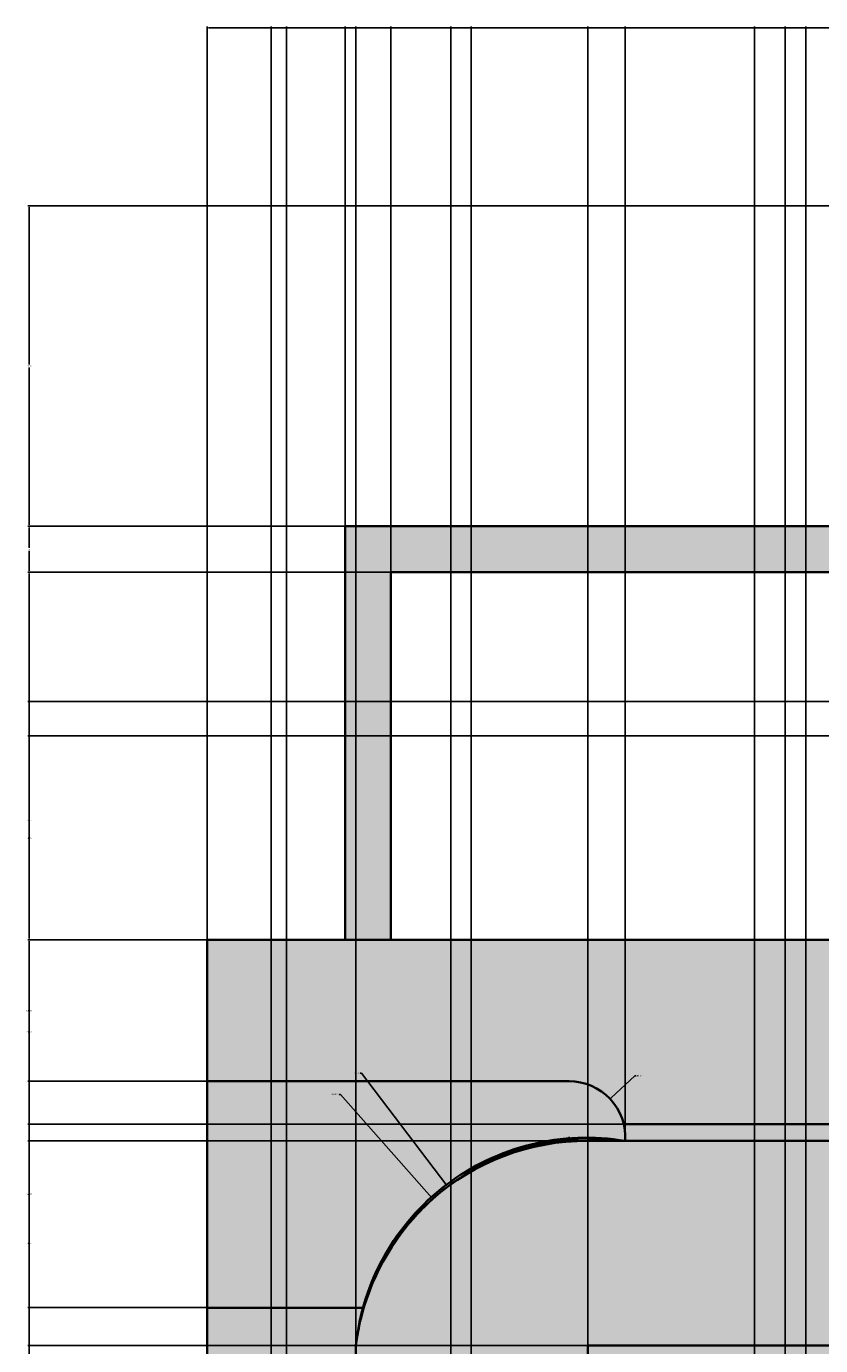
# Model space of a CAD drawing. Units: feet. Extents: x 2368 to 2738, y 1285 to 1782.
# Tile 3 of 6: x 2368 to 2472, y 1610 to 1782. Entities that reach past the tile are written whole.
import ezdxf

# ---------------------------------------------------------------- set-up
doc = ezdxf.new("R2010")
doc.units = ezdxf.units.FT
for name, color, linetype, lineweight in [('A-ANNO-DIMS', 2, 'Continuous', 18), ('A-ELEV', 7, 'Continuous', 35), ('A-ELEV-PATT', 252, 'Continuous', 13)]:
    doc.layers.add(name, color=color, linetype=linetype, lineweight=lineweight)
doc.styles.get("Standard").update_dxf_attribs({"font": 'arial.ttf'})
doc.dimstyles.get("Standard").update_dxf_attribs({"dimtxt": 0.18, "dimasz": 0.18, "dimexe": 0.18, "dimexo": 0.0625, "dimgap": 0.09, "dimtad": 0, "dimtih": 1, "dimtoh": 1, "dimdec": 1, "dimzin": 0, "dimdsep": 46, "dimlunit": 3, "dimtxsty": 'Standard', "dimcen": 0.09, "dimadec": 0, "dimazin": 0, "dimtfac": 1, "dimtdec": 1, "dimtofl": 0, "dimtmove": 0, "dimatfit": 3, "dimfxl": 1, "dimtolj": 1, "dimtzin": 0, "dimarcsym": 0})

# ---------------------------------------------------------------- blocks, each defined once
blk = doc.blocks.new('*D1')
at = {"layer": 'A-ANNO-DIMS', "color": 0, "lineweight": -2, "transparency": 16777216}
for p, q in [((2391.54, 1662.92), (2391.54, 1782.11)), ((2391.72, 1781.93), (2552.46, 1781.93)), ((2713.98, 1781.93), (2553.25, 1781.93)), ((2714.16, 1758.74), (2714.16, 1782.11))]:
    blk.add_line(p, q, dxfattribs=at)
at = {"layer": 'A-ANNO-DIMS', "color": 0, "transparency": 16777216}
for points in [[(2391.72, 1781.96), (2391.72, 1781.9), (2391.54, 1781.93)], [(2713.98, 1781.96), (2713.98, 1781.9), (2714.16, 1781.93)]]:
    blk.add_solid(points, dxfattribs=at)
at = {"layer": 'Defpoints', "color": 0, "transparency": 16777216}
for p in [(2714.16, 1781.93), (2714.16, 1758.68), (2391.54, 1662.86)]:
    blk.add_point(p, dxfattribs=at)
at = {"layer": 'A-ANNO-DIMS', "color": 0, "transparency": 16777216, "insert": (2552.85, 1781.93), "char_height": 0.18, "attachment_point": 5}
blk.add_mtext('\\A1;322.6', dxfattribs=at)
blk = doc.blocks.new('*D8')
at = {"layer": 'A-ANNO-DIMS', "color": 0, "lineweight": -2, "transparency": 16777216}
for p, q in [((2391.48, 1614.86), (2368.11, 1614.86)), ((2368.29, 1614.68), (2368.29, 1552.04)), ((2368.29, 1489.04), (2368.29, 1551.67)), ((2391.48, 1488.86), (2368.11, 1488.86))]:
    blk.add_line(p, q, dxfattribs=at)
at = {"layer": 'A-ANNO-DIMS', "color": 0, "transparency": 16777216}
for points in [[(2368.26, 1614.68), (2368.32, 1614.68), (2368.29, 1614.86)], [(2368.26, 1489.04), (2368.32, 1489.04), (2368.29, 1488.86)]]:
    blk.add_solid(points, dxfattribs=at)
at = {"layer": 'Defpoints', "color": 0, "transparency": 16777216}
for p in [(2368.29, 1614.86), (2391.54, 1614.86), (2391.54, 1488.86)]:
    blk.add_point(p, dxfattribs=at)
at = {"layer": 'A-ANNO-DIMS', "color": 0, "transparency": 16777216, "insert": (2368.29, 1551.86), "char_height": 0.18, "attachment_point": 5}
blk.add_mtext('\\A1;126', dxfattribs=at)
blk = doc.blocks.new('*D9')
at = {"layer": 'A-ANNO-DIMS', "color": 0, "lineweight": -2, "transparency": 16777216}
for p, q in [((2391.48, 1644.42), (2368.11, 1644.42)), ((2368.29, 1644.24), (2368.29, 1629.82)), ((2368.29, 1615.04), (2368.29, 1629.46)), ((2391.48, 1614.86), (2368.11, 1614.86))]:
    blk.add_line(p, q, dxfattribs=at)
at = {"layer": 'A-ANNO-DIMS', "color": 0, "transparency": 16777216}
for points in [[(2368.26, 1644.24), (2368.32, 1644.24), (2368.29, 1644.42)], [(2368.26, 1615.04), (2368.32, 1615.04), (2368.29, 1614.86)]]:
    blk.add_solid(points, dxfattribs=at)
at = {"layer": 'Defpoints', "color": 0, "transparency": 16777216}
for p in [(2368.29, 1644.42), (2391.54, 1644.42), (2391.54, 1614.86)]:
    blk.add_point(p, dxfattribs=at)
at = {"layer": 'A-ANNO-DIMS', "color": 0, "transparency": 16777216, "insert": (2368.29, 1629.64), "char_height": 0.18, "attachment_point": 5}
blk.add_mtext('\\A1;29.565', dxfattribs=at)
blk = doc.blocks.new('*D10')
at = {"layer": 'A-ANNO-DIMS', "color": 0, "lineweight": -2, "transparency": 16777216}
for p, q in [((2391.48, 1662.86), (2368.11, 1662.86)), ((2368.29, 1662.68), (2368.29, 1653.82)), ((2368.29, 1644.6), (2368.29, 1653.46)), ((2391.48, 1644.42), (2368.11, 1644.42))]:
    blk.add_line(p, q, dxfattribs=at)
at = {"layer": 'A-ANNO-DIMS', "color": 0, "transparency": 16777216}
for points in [[(2368.26, 1662.68), (2368.32, 1662.68), (2368.29, 1662.86)], [(2368.26, 1644.6), (2368.32, 1644.6), (2368.29, 1644.42)]]:
    blk.add_solid(points, dxfattribs=at)
at = {"layer": 'Defpoints', "color": 0, "transparency": 16777216}
for p in [(2368.29, 1662.86), (2391.54, 1662.86), (2391.54, 1644.42)]:
    blk.add_point(p, dxfattribs=at)
at = {"layer": 'A-ANNO-DIMS', "color": 0, "transparency": 16777216, "insert": (2368.29, 1653.64), "char_height": 0.18, "attachment_point": 5}
blk.add_mtext('\\A1;18.435', dxfattribs=at)
blk = doc.blocks.new('*D11')
at = {"layer": 'A-ANNO-DIMS', "color": 0, "lineweight": -2, "transparency": 16777216}
for p, q in [((2415.48, 1710.86), (2368.11, 1710.86)), ((2368.29, 1710.68), (2368.29, 1687.04)), ((2368.29, 1663.04), (2368.29, 1686.67)), ((2409.48, 1662.86), (2368.11, 1662.86))]:
    blk.add_line(p, q, dxfattribs=at)
at = {"layer": 'A-ANNO-DIMS', "color": 0, "transparency": 16777216}
for points in [[(2368.26, 1710.68), (2368.32, 1710.68), (2368.29, 1710.86)], [(2368.26, 1663.04), (2368.32, 1663.04), (2368.29, 1662.86)]]:
    blk.add_solid(points, dxfattribs=at)
at = {"layer": 'Defpoints', "color": 0, "transparency": 16777216}
for p in [(2368.29, 1710.86), (2415.54, 1710.86), (2409.54, 1662.86)]:
    blk.add_point(p, dxfattribs=at)
at = {"layer": 'A-ANNO-DIMS', "color": 0, "transparency": 16777216, "insert": (2368.29, 1686.86), "char_height": 0.18, "attachment_point": 5}
blk.add_mtext('\\A1;48', dxfattribs=at)
blk = doc.blocks.new('*D12')
at = {"layer": 'A-ANNO-DIMS', "color": 0, "lineweight": -2, "transparency": 16777216}
for p, q in [((2409.48, 1716.86), (2368.11, 1716.86)), ((2368.29, 1716.68), (2368.29, 1714.04)), ((2368.29, 1711.04), (2368.29, 1713.67)), ((2415.48, 1710.86), (2368.11, 1710.86))]:
    blk.add_line(p, q, dxfattribs=at)
at = {"layer": 'A-ANNO-DIMS', "color": 0, "transparency": 16777216}
for points in [[(2368.26, 1716.68), (2368.32, 1716.68), (2368.29, 1716.86)], [(2368.26, 1711.04), (2368.32, 1711.04), (2368.29, 1710.86)]]:
    blk.add_solid(points, dxfattribs=at)
at = {"layer": 'Defpoints', "color": 0, "transparency": 16777216}
for p in [(2368.29, 1716.86), (2409.54, 1716.86), (2415.54, 1710.86)]:
    blk.add_point(p, dxfattribs=at)
at = {"layer": 'A-ANNO-DIMS', "color": 0, "transparency": 16777216, "insert": (2368.29, 1713.86), "char_height": 0.18, "attachment_point": 5}
blk.add_mtext('\\A1;6', dxfattribs=at)
blk = doc.blocks.new('*D13')
at = {"layer": 'A-ANNO-DIMS', "color": 0, "lineweight": -2, "transparency": 16777216}
for p, q in [((2519.56, 1758.68), (2368.11, 1758.68)), ((2368.29, 1758.5), (2368.29, 1737.95)), ((2368.29, 1717.04), (2368.29, 1737.58)), ((2519.56, 1716.86), (2368.11, 1716.86))]:
    blk.add_line(p, q, dxfattribs=at)
at = {"layer": 'A-ANNO-DIMS', "color": 0, "transparency": 16777216}
for points in [[(2368.26, 1758.5), (2368.32, 1758.5), (2368.29, 1758.68)], [(2368.26, 1717.04), (2368.32, 1717.04), (2368.29, 1716.86)]]:
    blk.add_solid(points, dxfattribs=at)
at = {"layer": 'Defpoints', "color": 0, "transparency": 16777216}
for p in [(2368.29, 1758.68), (2519.62, 1758.68), (2519.62, 1716.86)]:
    blk.add_point(p, dxfattribs=at)
at = {"layer": 'A-ANNO-DIMS', "color": 0, "transparency": 16777216, "insert": (2368.29, 1737.77), "char_height": 0.18, "attachment_point": 5}
blk.add_mtext('\\A1;41.82', dxfattribs=at)
blk = doc.blocks.new('*D24')
at = {"layer": 'A-ANNO-DIMS', "color": 0, "lineweight": -2, "transparency": 16777216}
for p, q in [((2399.91, 1456.15), (2399.91, 1782.11)), ((2400.09, 1781.93), (2400.76, 1781.93)), ((2401.73, 1781.93), (2401.06, 1781.93)), ((2401.91, 1454.15), (2401.91, 1782.11))]:
    blk.add_line(p, q, dxfattribs=at)
at = {"layer": 'A-ANNO-DIMS', "color": 0, "transparency": 16777216}
for points in [[(2400.09, 1781.96), (2400.09, 1781.9), (2399.91, 1781.93)], [(2401.73, 1781.96), (2401.73, 1781.9), (2401.91, 1781.93)]]:
    blk.add_solid(points, dxfattribs=at)
at = {"layer": 'Defpoints', "color": 0, "transparency": 16777216}
for p in [(2401.91, 1781.93), (2399.91, 1456.08), (2401.91, 1454.08)]:
    blk.add_point(p, dxfattribs=at)
at = {"layer": 'A-ANNO-DIMS', "color": 0, "transparency": 16777216, "insert": (2400.91, 1781.93), "char_height": 0.18, "attachment_point": 5}
blk.add_mtext('\\A1;2', dxfattribs=at)
blk = doc.blocks.new('*D30')
at = {"layer": 'A-ANNO-DIMS', "color": 0, "lineweight": -2, "transparency": 16777216}
for p, q in [((2463.03, 1460.16), (2463.03, 1782.11)), ((2463.21, 1781.93), (2464.88, 1781.93)), ((2466.85, 1781.93), (2465.18, 1781.93)), ((2467.03, 1456.16), (2467.03, 1782.11))]:
    blk.add_line(p, q, dxfattribs=at)
at = {"layer": 'A-ANNO-DIMS', "color": 0, "transparency": 16777216}
for points in [[(2463.21, 1781.96), (2463.21, 1781.9), (2463.03, 1781.93)], [(2466.85, 1781.96), (2466.85, 1781.9), (2467.03, 1781.93)]]:
    blk.add_solid(points, dxfattribs=at)
at = {"layer": 'Defpoints', "color": 0, "transparency": 16777216}
for p in [(2467.03, 1781.93), (2463.03, 1460.1), (2467.03, 1456.1)]:
    blk.add_point(p, dxfattribs=at)
at = {"layer": 'A-ANNO-DIMS', "color": 0, "transparency": 16777216, "insert": (2465.03, 1781.93), "char_height": 0.18, "attachment_point": 5}
blk.add_mtext('\\A1;4', dxfattribs=at)
blk = doc.blocks.new('*D38')
at = {"layer": 'A-ANNO-DIMS', "color": 0, "lineweight": -2, "transparency": 16777216}
for p, q in [((2701.6, 1636.62), (2368.11, 1636.62)), ((2368.29, 1636.44), (2368.29, 1623.45)), ((2368.29, 1610.09), (2368.29, 1623.08)), ((2701.6, 1609.91), (2368.11, 1609.91))]:
    blk.add_line(p, q, dxfattribs=at)
at = {"layer": 'A-ANNO-DIMS', "color": 0, "transparency": 16777216}
for points in [[(2368.26, 1636.44), (2368.32, 1636.44), (2368.29, 1636.62)], [(2368.26, 1610.09), (2368.32, 1610.09), (2368.29, 1609.91)]]:
    blk.add_solid(points, dxfattribs=at)
at = {"layer": 'Defpoints', "color": 0, "transparency": 16777216}
for p in [(2368.29, 1636.62), (2701.66, 1636.62), (2701.66, 1609.91)]:
    blk.add_point(p, dxfattribs=at)
at = {"layer": 'A-ANNO-DIMS', "color": 0, "transparency": 16777216, "insert": (2368.29, 1623.26), "char_height": 0.18, "attachment_point": 5}
blk.add_mtext('\\A1;26.72', dxfattribs=at)
blk = doc.blocks.new('*D39')
at = {"layer": 'A-ANNO-DIMS', "color": 0, "lineweight": -2, "transparency": 16777216}
for p, q in [((2701.6, 1662.86), (2368.11, 1662.86)), ((2368.29, 1662.68), (2368.29, 1651.02)), ((2368.29, 1638.99), (2368.29, 1650.65)), ((2701.6, 1638.81), (2368.11, 1638.81))]:
    blk.add_line(p, q, dxfattribs=at)
at = {"layer": 'A-ANNO-DIMS', "color": 0, "transparency": 16777216}
for points in [[(2368.26, 1662.68), (2368.32, 1662.68), (2368.29, 1662.86)], [(2368.26, 1638.99), (2368.32, 1638.99), (2368.29, 1638.81)]]:
    blk.add_solid(points, dxfattribs=at)
at = {"layer": 'Defpoints', "color": 0, "transparency": 16777216}
for p in [(2368.29, 1662.86), (2701.66, 1662.86), (2701.66, 1638.81)]:
    blk.add_point(p, dxfattribs=at)
at = {"layer": 'A-ANNO-DIMS', "color": 0, "transparency": 16777216, "insert": (2368.29, 1650.83), "char_height": 0.18, "attachment_point": 5}
blk.add_mtext('\\A1;24.042', dxfattribs=at)
blk = doc.blocks.new('*D40')
at = {"layer": 'A-ANNO-DIMS', "color": 0, "lineweight": -2, "transparency": 16777216}
for p, q in [((2701.6, 1693.98), (2368.11, 1693.98)), ((2368.29, 1693.8), (2368.29, 1678.6)), ((2368.29, 1663.04), (2368.29, 1678.24)), ((2701.6, 1662.86), (2368.11, 1662.86))]:
    blk.add_line(p, q, dxfattribs=at)
at = {"layer": 'A-ANNO-DIMS', "color": 0, "transparency": 16777216}
for points in [[(2368.26, 1693.8), (2368.32, 1693.8), (2368.29, 1693.98)], [(2368.26, 1663.04), (2368.32, 1663.04), (2368.29, 1662.86)]]:
    blk.add_solid(points, dxfattribs=at)
at = {"layer": 'Defpoints', "color": 0, "transparency": 16777216}
for p in [(2368.29, 1693.98), (2701.66, 1693.98), (2701.66, 1662.86)]:
    blk.add_point(p, dxfattribs=at)
at = {"layer": 'A-ANNO-DIMS', "color": 0, "transparency": 16777216, "insert": (2368.29, 1678.42), "char_height": 0.18, "attachment_point": 5}
blk.add_mtext('\\A1;31.13', dxfattribs=at)
blk = doc.blocks.new('*D41')
at = {"layer": 'A-ANNO-DIMS', "color": 0, "lineweight": -2, "transparency": 16777216}
for p, q in [((2391.54, 1488.92), (2391.54, 1782.11)), ((2391.72, 1781.93), (2400.79, 1781.93)), ((2410.77, 1781.93), (2401.7, 1781.93)), ((2410.95, 1488.92), (2410.95, 1782.11))]:
    blk.add_line(p, q, dxfattribs=at)
at = {"layer": 'A-ANNO-DIMS', "color": 0, "transparency": 16777216}
for points in [[(2391.72, 1781.96), (2391.72, 1781.9), (2391.54, 1781.93)], [(2410.77, 1781.96), (2410.77, 1781.9), (2410.95, 1781.93)]]:
    blk.add_solid(points, dxfattribs=at)
at = {"layer": 'Defpoints', "color": 0, "transparency": 16777216}
for p in [(2410.95, 1781.93), (2391.54, 1488.86), (2410.95, 1488.86)]:
    blk.add_point(p, dxfattribs=at)
at = {"layer": 'A-ANNO-DIMS', "color": 0, "transparency": 16777216, "insert": (2401.24, 1781.93), "char_height": 0.18, "attachment_point": 5}
blk.add_mtext('\\A1;19.406', dxfattribs=at)
blk = doc.blocks.new('*D42')
at = {"layer": 'A-ANNO-DIMS', "color": 0, "lineweight": -2, "transparency": 16777216}
for p, q in [((2410.88, 1609.91), (2368.11, 1609.91)), ((2368.29, 1609.73), (2368.29, 1549.56)), ((2368.29, 1489.04), (2368.29, 1549.2)), ((2410.88, 1488.86), (2368.11, 1488.86))]:
    blk.add_line(p, q, dxfattribs=at)
at = {"layer": 'A-ANNO-DIMS', "color": 0, "transparency": 16777216}
for points in [[(2368.26, 1609.73), (2368.32, 1609.73), (2368.29, 1609.91)], [(2368.26, 1489.04), (2368.32, 1489.04), (2368.29, 1488.86)]]:
    blk.add_solid(points, dxfattribs=at)
at = {"layer": 'Defpoints', "color": 0, "transparency": 16777216}
for p in [(2368.29, 1609.91), (2410.95, 1609.91), (2410.95, 1488.86)]:
    blk.add_point(p, dxfattribs=at)
at = {"layer": 'A-ANNO-DIMS', "color": 0, "transparency": 16777216, "insert": (2368.29, 1549.38), "char_height": 0.18, "attachment_point": 5}
blk.add_mtext('\\A1;121.05', dxfattribs=at)
blk = doc.blocks.new('*D43')
at = {"layer": 'A-ANNO-DIMS', "color": 0, "lineweight": -2, "transparency": 16777216}
for p, q in [((2410.95, 1609.97), (2410.95, 1782.11)), ((2411.13, 1781.93), (2416.69, 1781.93)), ((2423.16, 1781.93), (2417.6, 1781.93)), ((2423.34, 1606.5), (2423.34, 1782.11))]:
    blk.add_line(p, q, dxfattribs=at)
at = {"layer": 'A-ANNO-DIMS', "color": 0, "transparency": 16777216}
for points in [[(2411.13, 1781.96), (2411.13, 1781.9), (2410.95, 1781.93)], [(2423.16, 1781.96), (2423.16, 1781.9), (2423.34, 1781.93)]]:
    blk.add_solid(points, dxfattribs=at)
at = {"layer": 'Defpoints', "color": 0, "transparency": 16777216}
for p in [(2423.34, 1781.93), (2410.95, 1609.91), (2423.34, 1606.44)]:
    blk.add_point(p, dxfattribs=at)
at = {"layer": 'A-ANNO-DIMS', "color": 0, "transparency": 16777216, "insert": (2417.15, 1781.93), "char_height": 0.18, "attachment_point": 5}
blk.add_mtext('\\A1;12.396', dxfattribs=at)
blk = doc.blocks.new('*D44')
at = {"layer": 'A-ANNO-DIMS', "color": 0, "lineweight": -2, "transparency": 16777216}
for p, q in [((2423.34, 1606.5), (2423.34, 1782.11)), ((2423.52, 1781.93), (2424.36, 1781.93)), ((2425.85, 1781.93), (2425.01, 1781.93)), ((2426.03, 1606.5), (2426.03, 1782.11))]:
    blk.add_line(p, q, dxfattribs=at)
at = {"layer": 'A-ANNO-DIMS', "color": 0, "transparency": 16777216}
for points in [[(2423.52, 1781.96), (2423.52, 1781.9), (2423.34, 1781.93)], [(2425.85, 1781.96), (2425.85, 1781.9), (2426.03, 1781.93)]]:
    blk.add_solid(points, dxfattribs=at)
at = {"layer": 'Defpoints', "color": 0, "transparency": 16777216}
for p in [(2426.03, 1781.93), (2423.34, 1606.44), (2426.03, 1606.44)]:
    blk.add_point(p, dxfattribs=at)
at = {"layer": 'A-ANNO-DIMS', "color": 0, "transparency": 16777216, "insert": (2424.69, 1781.93), "char_height": 0.18, "attachment_point": 5}
blk.add_mtext('\\A1;2.69', dxfattribs=at)
blk = doc.blocks.new('*D45')
at = {"layer": 'A-ANNO-DIMS', "color": 0, "lineweight": -2, "transparency": 16777216}
for p, q in [((2426.03, 1606.5), (2426.03, 1782.11)), ((2426.21, 1781.93), (2433.19, 1781.93)), ((2441.07, 1781.93), (2434.1, 1781.93)), ((2441.25, 1609.97), (2441.25, 1782.11))]:
    blk.add_line(p, q, dxfattribs=at)
at = {"layer": 'A-ANNO-DIMS', "color": 0, "transparency": 16777216}
for points in [[(2426.21, 1781.96), (2426.21, 1781.9), (2426.03, 1781.93)], [(2441.07, 1781.96), (2441.07, 1781.9), (2441.25, 1781.93)]]:
    blk.add_solid(points, dxfattribs=at)
at = {"layer": 'Defpoints', "color": 0, "transparency": 16777216}
for p in [(2441.25, 1781.93), (2441.25, 1609.91), (2426.03, 1606.44)]:
    blk.add_point(p, dxfattribs=at)
at = {"layer": 'A-ANNO-DIMS', "color": 0, "transparency": 16777216, "insert": (2433.64, 1781.93), "char_height": 0.18, "attachment_point": 5}
blk.add_mtext('\\A1;15.216', dxfattribs=at)
blk = doc.blocks.new('*D49')
at = {"layer": 'A-ANNO-DIMS', "color": 0, "lineweight": -2, "transparency": 16777216}
for p, q in [((2441.19, 1609.91), (2368.11, 1609.91)), ((2368.29, 1609.73), (2368.29, 1564.99)), ((2368.29, 1519.89), (2368.29, 1564.63)), ((2441.19, 1519.71), (2368.11, 1519.71))]:
    blk.add_line(p, q, dxfattribs=at)
at = {"layer": 'A-ANNO-DIMS', "color": 0, "transparency": 16777216}
for points in [[(2368.26, 1609.73), (2368.32, 1609.73), (2368.29, 1609.91)], [(2368.26, 1519.89), (2368.32, 1519.89), (2368.29, 1519.71)]]:
    blk.add_solid(points, dxfattribs=at)
at = {"layer": 'Defpoints', "color": 0, "transparency": 16777216}
for p in [(2368.29, 1609.91), (2441.25, 1609.91), (2441.25, 1519.71)]:
    blk.add_point(p, dxfattribs=at)
at = {"layer": 'A-ANNO-DIMS', "color": 0, "transparency": 16777216, "insert": (2368.29, 1564.81), "char_height": 0.18, "attachment_point": 5}
blk.add_mtext('\\A1;90.2', dxfattribs=at)
blk = doc.blocks.new('*D50')
at = {"layer": 'A-ANNO-DIMS', "color": 0, "lineweight": -2, "transparency": 16777216}
for p, q in [((2441.25, 1519.77), (2441.25, 1782.11)), ((2441.43, 1781.93), (2455.03, 1781.93)), ((2469.55, 1781.93), (2455.96, 1781.93)), ((2469.73, 1519.4), (2469.73, 1782.11))]:
    blk.add_line(p, q, dxfattribs=at)
at = {"layer": 'A-ANNO-DIMS', "color": 0, "transparency": 16777216}
for points in [[(2441.43, 1781.96), (2441.43, 1781.9), (2441.25, 1781.93)], [(2469.55, 1781.96), (2469.55, 1781.9), (2469.73, 1781.93)]]:
    blk.add_solid(points, dxfattribs=at)
at = {"layer": 'Defpoints', "color": 0, "transparency": 16777216}
for p in [(2469.73, 1781.93), (2441.25, 1519.71), (2469.73, 1519.33)]:
    blk.add_point(p, dxfattribs=at)
at = {"layer": 'A-ANNO-DIMS', "color": 0, "transparency": 16777216, "insert": (2455.49, 1781.93), "char_height": 0.18, "attachment_point": 5}
blk.add_mtext('\\A1;28.486', dxfattribs=at)
blk = doc.blocks.new('*D52')
at = {"layer": 'A-ANNO-DIMS', "color": 0, "lineweight": -2, "transparency": 16777216}
for p, q in [((2463.03, 1598.16), (2463.03, 1782.11)), ((2463.21, 1781.93), (2464.88, 1781.93)), ((2466.85, 1781.93), (2465.18, 1781.93)), ((2467.03, 1594.16), (2467.03, 1782.11))]:
    blk.add_line(p, q, dxfattribs=at)
at = {"layer": 'A-ANNO-DIMS', "color": 0, "transparency": 16777216}
for points in [[(2463.21, 1781.96), (2463.21, 1781.9), (2463.03, 1781.93)], [(2466.85, 1781.96), (2466.85, 1781.9), (2467.03, 1781.93)]]:
    blk.add_solid(points, dxfattribs=at)
at = {"layer": 'Defpoints', "color": 0, "transparency": 16777216}
for p in [(2467.03, 1781.93), (2463.03, 1598.1), (2467.03, 1594.1)]:
    blk.add_point(p, dxfattribs=at)
at = {"layer": 'A-ANNO-DIMS', "color": 0, "transparency": 16777216, "insert": (2465.03, 1781.93), "char_height": 0.18, "attachment_point": 5}
blk.add_mtext('\\A1;4', dxfattribs=at)
blk = doc.blocks.new('*D53')
at = {"layer": 'A-ANNO-DIMS', "color": 0, "lineweight": -2, "transparency": 16777216}
for p, q in [((2441.25, 1609.97), (2441.25, 1782.11)), ((2441.43, 1781.93), (2500.56, 1781.93)), ((2560.6, 1781.93), (2501.47, 1781.93)), ((2560.78, 1609.97), (2560.78, 1782.11))]:
    blk.add_line(p, q, dxfattribs=at)
at = {"layer": 'A-ANNO-DIMS', "color": 0, "transparency": 16777216}
for points in [[(2441.43, 1781.96), (2441.43, 1781.9), (2441.25, 1781.93)], [(2560.6, 1781.96), (2560.6, 1781.9), (2560.78, 1781.93)]]:
    blk.add_solid(points, dxfattribs=at)
at = {"layer": 'Defpoints', "color": 0, "transparency": 16777216}
for p in [(2560.78, 1781.93), (2441.25, 1609.91), (2560.78, 1609.91)]:
    blk.add_point(p, dxfattribs=at)
at = {"layer": 'A-ANNO-DIMS', "color": 0, "transparency": 16777216, "insert": (2501.01, 1781.93), "char_height": 0.18, "attachment_point": 5}
blk.add_mtext('\\A1;119.53', dxfattribs=at)
blk = doc.blocks.new('*D61')
at = {"layer": 'A-ANNO-DIMS', "color": 0, "lineweight": -2, "transparency": 16777216}
for p, q in [((2391.54, 1644.48), (2391.54, 1782.11)), ((2391.72, 1781.93), (2418.52, 1781.93)), ((2445.96, 1781.93), (2419.17, 1781.93)), ((2446.14, 1636.69), (2446.14, 1782.11))]:
    blk.add_line(p, q, dxfattribs=at)
at = {"layer": 'A-ANNO-DIMS', "color": 0, "transparency": 16777216}
for points in [[(2391.72, 1781.96), (2391.72, 1781.9), (2391.54, 1781.93)], [(2445.96, 1781.96), (2445.96, 1781.9), (2446.14, 1781.93)]]:
    blk.add_solid(points, dxfattribs=at)
at = {"layer": 'Defpoints', "color": 0, "transparency": 16777216}
for p in [(2446.14, 1781.93), (2391.54, 1644.42), (2446.14, 1636.62)]:
    blk.add_point(p, dxfattribs=at)
at = {"layer": 'A-ANNO-DIMS', "color": 0, "transparency": 16777216, "insert": (2418.84, 1781.93), "char_height": 0.18, "attachment_point": 5}
blk.add_mtext('\\A1;54.6', dxfattribs=at)
blk = doc.blocks.new('*D62')
at = {"layer": 'A-ANNO-DIMS', "color": 0, "lineweight": -2, "transparency": 16777216}
for p, q in [((2441.25, 1636.69), (2441.25, 1782.11)), ((2441.43, 1781.93), (2491.36, 1781.93)), ((2542.19, 1781.93), (2492.27, 1781.93)), ((2542.37, 1636.69), (2542.37, 1782.11))]:
    blk.add_line(p, q, dxfattribs=at)
at = {"layer": 'A-ANNO-DIMS', "color": 0, "transparency": 16777216}
for points in [[(2441.43, 1781.96), (2441.43, 1781.9), (2441.25, 1781.93)], [(2542.19, 1781.96), (2542.19, 1781.9), (2542.37, 1781.93)]]:
    blk.add_solid(points, dxfattribs=at)
at = {"layer": 'Defpoints', "color": 0, "transparency": 16777216}
for p in [(2542.37, 1781.93), (2441.25, 1636.62), (2542.37, 1636.62)]:
    blk.add_point(p, dxfattribs=at)
at = {"layer": 'A-ANNO-DIMS', "color": 0, "transparency": 16777216, "insert": (2491.81, 1781.93), "char_height": 0.18, "attachment_point": 5}
blk.add_mtext('\\A1;101.13', dxfattribs=at)
blk = doc.blocks.new('*D63')
at = {"layer": 'A-ANNO-DIMS', "color": 0, "lineweight": -2, "transparency": 16777216}
for p, q in [((2415.54, 1662.92), (2415.54, 1782.11)), ((2415.72, 1781.93), (2460.47, 1781.93)), ((2506.02, 1781.93), (2461.26, 1781.93)), ((2506.2, 1662.92), (2506.2, 1782.11))]:
    blk.add_line(p, q, dxfattribs=at)
at = {"layer": 'A-ANNO-DIMS', "color": 0, "transparency": 16777216}
for points in [[(2415.72, 1781.96), (2415.72, 1781.9), (2415.54, 1781.93)], [(2506.02, 1781.96), (2506.02, 1781.9), (2506.2, 1781.93)]]:
    blk.add_solid(points, dxfattribs=at)
at = {"layer": 'Defpoints', "color": 0, "transparency": 16777216}
for p in [(2506.2, 1781.93), (2415.54, 1662.86), (2506.2, 1662.86)]:
    blk.add_point(p, dxfattribs=at)
at = {"layer": 'A-ANNO-DIMS', "color": 0, "transparency": 16777216, "insert": (2460.87, 1781.93), "char_height": 0.18, "attachment_point": 5}
blk.add_mtext('\\A1;90.65', dxfattribs=at)
blk = doc.blocks.new('*D66')
at = {"layer": 'A-ANNO-DIMS', "color": 0, "lineweight": -2, "transparency": 16777216}
for p, q in [((2391.54, 1662.92), (2391.54, 1782.11)), ((2391.72, 1781.93), (2400.33, 1781.93)), ((2409.36, 1781.93), (2400.75, 1781.93)), ((2409.54, 1662.92), (2409.54, 1782.11))]:
    blk.add_line(p, q, dxfattribs=at)
at = {"layer": 'A-ANNO-DIMS', "color": 0, "transparency": 16777216}
for points in [[(2391.72, 1781.96), (2391.72, 1781.9), (2391.54, 1781.93)], [(2409.36, 1781.96), (2409.36, 1781.9), (2409.54, 1781.93)]]:
    blk.add_solid(points, dxfattribs=at)
at = {"layer": 'Defpoints', "color": 0, "transparency": 16777216}
for p in [(2409.54, 1781.93), (2391.54, 1662.86), (2409.54, 1662.86)]:
    blk.add_point(p, dxfattribs=at)
at = {"layer": 'A-ANNO-DIMS', "color": 0, "transparency": 16777216, "insert": (2400.54, 1781.93), "char_height": 0.18, "attachment_point": 5}
blk.add_mtext('\\A1;18', dxfattribs=at)
blk = doc.blocks.new('*D67')
at = {"layer": 'A-ANNO-DIMS', "color": 0, "lineweight": -2, "transparency": 16777216}
for p, q in [((2409.54, 1662.92), (2409.54, 1782.11)), ((2409.72, 1781.93), (2412.39, 1781.93)), ((2415.36, 1781.93), (2412.69, 1781.93)), ((2415.54, 1662.92), (2415.54, 1782.11))]:
    blk.add_line(p, q, dxfattribs=at)
at = {"layer": 'A-ANNO-DIMS', "color": 0, "transparency": 16777216}
for points in [[(2409.72, 1781.96), (2409.72, 1781.9), (2409.54, 1781.93)], [(2415.36, 1781.96), (2415.36, 1781.9), (2415.54, 1781.93)]]:
    blk.add_solid(points, dxfattribs=at)
at = {"layer": 'Defpoints', "color": 0, "transparency": 16777216}
for p in [(2415.54, 1781.93), (2409.54, 1662.86), (2415.54, 1662.86)]:
    blk.add_point(p, dxfattribs=at)
at = {"layer": 'A-ANNO-DIMS', "color": 0, "transparency": 16777216, "insert": (2412.54, 1781.93), "char_height": 0.18, "attachment_point": 5}
blk.add_mtext('\\A1;6', dxfattribs=at)
blk = doc.blocks.new('*D68')
at = {"layer": 'A-ANNO-DIMS', "color": 0, "lineweight": -2, "transparency": 16777216}
for p, q in [((2409.54, 1716.92), (2409.54, 1782.11)), ((2409.72, 1781.93), (2464.13, 1781.93)), ((2519.44, 1781.93), (2465.04, 1781.93)), ((2519.62, 1716.92), (2519.62, 1782.11))]:
    blk.add_line(p, q, dxfattribs=at)
at = {"layer": 'A-ANNO-DIMS', "color": 0, "transparency": 16777216}
for points in [[(2409.72, 1781.96), (2409.72, 1781.9), (2409.54, 1781.93)], [(2519.44, 1781.96), (2519.44, 1781.9), (2519.62, 1781.93)]]:
    blk.add_solid(points, dxfattribs=at)
at = {"layer": 'Defpoints', "color": 0, "transparency": 16777216}
for p in [(2519.62, 1781.93), (2409.54, 1716.86), (2519.62, 1716.86)]:
    blk.add_point(p, dxfattribs=at)
at = {"layer": 'A-ANNO-DIMS', "color": 0, "transparency": 16777216, "insert": (2464.58, 1781.93), "char_height": 0.18, "attachment_point": 5}
blk.add_mtext('\\A1;110.08', dxfattribs=at)
blk = doc.blocks.new('*D71')
at = {"layer": 'A-ANNO-DIMS', "color": 0, "lineweight": -2, "transparency": 16777216}
for p, q in [((2592.35, 1689.49), (2368.11, 1689.49)), ((2368.29, 1689.31), (2368.29, 1676.36)), ((2368.29, 1663.04), (2368.29, 1675.99)), ((2592.35, 1662.86), (2368.11, 1662.86))]:
    blk.add_line(p, q, dxfattribs=at)
at = {"layer": 'A-ANNO-DIMS', "color": 0, "transparency": 16777216}
for points in [[(2368.26, 1689.31), (2368.32, 1689.31), (2368.29, 1689.49)], [(2368.26, 1663.04), (2368.32, 1663.04), (2368.29, 1662.86)]]:
    blk.add_solid(points, dxfattribs=at)
at = {"layer": 'Defpoints', "color": 0, "transparency": 16777216}
for p in [(2368.29, 1689.49), (2592.41, 1689.49), (2592.41, 1662.86)]:
    blk.add_point(p, dxfattribs=at)
at = {"layer": 'A-ANNO-DIMS', "color": 0, "transparency": 16777216, "insert": (2368.29, 1676.17), "char_height": 0.18, "attachment_point": 5}
blk.add_mtext('\\A1;26.64', dxfattribs=at)
blk = doc.blocks.new('*D74')
at = {"layer": 'A-ANNO-DIMS', "color": 0, "lineweight": -2, "transparency": 16777216}
for p, q in [((2411.53, 1645.45), (2411.71, 1645.45)), ((2411.71, 1645.45), (2422.83, 1630.8)), ((2441.56, 1606), (2441.74, 1606)), ((2441.65, 1605.91), (2441.65, 1606.09))]:
    blk.add_line(p, q, dxfattribs=at)
at = {"layer": 'A-ANNO-DIMS', "color": 0, "transparency": 16777216}
blk.add_solid([(2422.85, 1630.81), (2422.8, 1630.78), (2422.94, 1630.65)], dxfattribs=at)
at = {"layer": 'Defpoints', "color": 0, "transparency": 16777216}
for p in [(2422.94, 1630.65), (2441.65, 1606)]:
    blk.add_point(p, dxfattribs=at)
at = {"layer": 'A-ANNO-DIMS', "color": 0, "transparency": 16777216, "insert": (2411.05, 1645.45), "char_height": 0.18, "attachment_point": 5}
blk.add_mtext('\\A1;R30.95', dxfattribs=at)
blk = doc.blocks.new('*D75')
at = {"layer": 'A-ANNO-DIMS', "color": 0, "lineweight": -2, "transparency": 16777216}
for p, q in [((2447.38, 1645.12), (2444.3, 1642.23)), ((2447.56, 1645.12), (2447.38, 1645.12)), ((2438.73, 1637.08), (2438.91, 1637.08)), ((2438.82, 1636.99), (2438.82, 1637.17))]:
    blk.add_line(p, q, dxfattribs=at)
at = {"layer": 'A-ANNO-DIMS', "color": 0, "transparency": 16777216}
blk.add_solid([(2444.28, 1642.25), (2444.32, 1642.21), (2444.17, 1642.11)], dxfattribs=at)
at = {"layer": 'Defpoints', "color": 0, "transparency": 16777216}
for p in [(2444.17, 1642.11), (2438.82, 1637.08)]:
    blk.add_point(p, dxfattribs=at)
at = {"layer": 'A-ANNO-DIMS', "color": 0, "transparency": 16777216, "insert": (2448.04, 1645.12), "char_height": 0.18, "attachment_point": 5}
blk.add_mtext('\\A1;R7.344', dxfattribs=at)
blk = doc.blocks.new('*D76')
at = {"layer": 'A-ANNO-DIMS', "color": 0, "lineweight": -2, "transparency": 16777216}
for p, q in [((2408.79, 1642.69), (2408.97, 1642.69)), ((2408.97, 1642.69), (2420.88, 1629.19)), ((2440.95, 1606.32), (2441.13, 1606.32)), ((2441.04, 1606.23), (2441.04, 1606.41))]:
    blk.add_line(p, q, dxfattribs=at)
at = {"layer": 'A-ANNO-DIMS', "color": 0, "transparency": 16777216}
blk.add_solid([(2420.9, 1629.21), (2420.85, 1629.17), (2421, 1629.05)], dxfattribs=at)
at = {"layer": 'Defpoints', "color": 0, "transparency": 16777216}
for p in [(2421, 1629.05), (2441.04, 1606.32)]:
    blk.add_point(p, dxfattribs=at)
at = {"layer": 'A-ANNO-DIMS', "color": 0, "transparency": 16777216, "insert": (2408.19, 1642.69), "char_height": 0.18, "attachment_point": 5}
blk.add_mtext('\\A1;2X R30.3', dxfattribs=at)

msp = doc.modelspace()

# ---------------------------------------------------------------- hatches: boundary and pattern name
at = {"layer": 'A-ELEV-PATT'}
h = msp.add_hatch(color=256, dxfattribs=at)
h.set_gradient(color1=(192, 192, 192), color2=(192, 192, 192), tint=1)
h.paths.add_polyline_path([(2714.1625, 1758.6751), (2519.621, 1758.6751), (2519.621, 1716.8552), (2714.1625, 1716.8552)])
h.paths.add_polyline_path([(2701.6591, 1693.9847), (2714.1625, 1693.9847), (2714.1625, 1710.8552), (2519.621, 1710.8552), (2519.621, 1662.8552), (2592.4132, 1662.8552), (2592.4132, 1689.493), (2665.1962, 1689.493), (2665.1962, 1662.8552), (2701.6591, 1662.8552)])
h.paths.add_polyline_path([(2701.6591, 1609.9058), (2597.776, 1609.9058), (2597.776, 1600.4784), (2665.1962, 1600.4784), (2665.1962, 1596.3371), (2665.1962, 1522.6314), (2701.6591, 1522.6314)])
h.paths.add_polyline_path([(2463.0324, 1598.097), (2536.677, 1598.097), (2536.677, 1519.7115), (2560.74, 1519.7115), (2560.5754, 1609.9058), (2542.3749, 1609.9058), (2441.2488, 1609.9058), (2441.2488, 1519.7115), (2463.0324, 1519.7115)])
h.paths.add_polyline_path([(2506.1956, 1662.8552), (2391.5414, 1662.8552), (2391.5414, 1644.4206), (2438.815, 1644.4206, -0.34592239), (2445.9507, 1638.8128), (2506.1956, 1638.8128)])
h.paths.add_polyline_path([(2410.9473, 1609.9058, -0.04175491), (2411.9608, 1614.8552), (2391.5414, 1614.8552), (2391.5414, 1488.8552), (2410.9473, 1488.8552)])
h.paths.add_polyline_path([(2426.5897, 1605.0962, 1), (2422.7862, 1605.0962), (2422.7862, 1509.5049, 1), (2426.5897, 1509.5049)])
h.paths.add_polyline_path([(2463.0324, 1460.097), (2536.677, 1460.097), (2536.677, 1350.8552), (2543.4468, 1350.8552), (2543.4468, 1482.8552), (2391.5414, 1482.8552), (2391.5414, 1350.8552), (2463.0324, 1350.8552)])
h.paths.add_polyline_path([(2436.8485, 1456.084), (2436.8485, 1379.669), (2399.9065, 1379.669), (2399.9065, 1456.084)], flags=16)
h.paths.add_polyline_path([(2434.8485, 1454.084), (2434.8485, 1381.669), (2401.9065, 1381.669), (2401.9065, 1454.084)], flags=0)
h.paths.add_polyline_path([(2714.1625, 1350.8552), (2391.5414, 1350.8552), (2391.5414, 1320.8552), (2714.1625, 1320.8552)])
h.paths.add_polyline_path([(2714.1625, 1320.8552), (2391.5414, 1320.8552), (2391.5414, 1308.8552), (2714.1625, 1308.8552)])
h = msp.add_hatch(color=256, dxfattribs=at)
h.set_gradient(color1=(128, 128, 128), color2=(128, 128, 128), tint=1)
h.paths.add_polyline_path([(2519.621, 1716.8552), (2409.5414, 1716.8552), (2409.5414, 1662.8552), (2415.5414, 1662.8552), (2415.5414, 1710.8552), (2519.621, 1710.8552)])
h.paths.add_polyline_path([(2714.1625, 1716.8552), (2519.621, 1716.8552), (2519.621, 1710.8552), (2714.1625, 1710.8552)])
h.paths.add_polyline_path([(2701.6591, 1638.8128), (2445.9507, 1638.8128, -0.0752442), (2446.1448, 1636.6235), (2542.3749, 1636.6235), (2542.776, 1636.6235), (2701.6591, 1636.6235)])
h = msp.add_hatch(color=256, dxfattribs=at)
h.set_gradient(color1=(242, 242, 242), color2=(242, 242, 242), tint=1)
h.paths.add_polyline_path([(2542.3749, 1636.6235), (2440.8236, 1636.6235, 0.37790365), (2410.9473, 1609.9058), (2410.9473, 1488.8552), (2441.2488, 1488.8552), (2441.2488, 1609.9058), (2542.3749, 1609.9058)])
h.paths.add_polyline_path([(2426.5897, 1605.0962), (2426.5897, 1509.5049, -1), (2422.7862, 1509.5049), (2422.7862, 1605.0962, -1)], flags=16)
h.paths.add_polyline_path([(2441.2488, 1636.6235), (2446.1448, 1636.6235, 0.43242195), (2438.815, 1644.4206), (2391.5414, 1644.4206), (2391.5414, 1620.8552), (2391.5414, 1614.8552), (2411.9608, 1614.8552, -0.33482359)])
h.paths.add_polyline_path([(2592.4132, 1461.1396), (2635.4878, 1461.1396), (2635.4878, 1466.101), (2560.7963, 1466.101), (2560.7963, 1482.8552), (2543.4468, 1482.8552), (2543.4468, 1350.8552), (2635.4878, 1350.8552), (2635.4878, 1367.9838), (2592.4132, 1367.9838)])
h = msp.add_hatch(color=256, dxfattribs=at)
h.set_gradient(color1=(205, 105, 40), color2=(205, 105, 40), tint=1)
h.paths.add_polyline_path([(2438.815, 1644.4206), (2391.5414, 1644.4206), (2391.5414, 1620.8552), (2391.5414, 1614.8552), (2411.887, 1614.8552, -0.3843416), (2446.1448, 1636.6235, 0.43242195)])

# ---------------------------------------------------------------- linework, layer by layer
at = {"layer": 'A-ELEV'}
for p, q in [((2409.5414, 1716.8552), (2409.5414, 1662.8552)), ((2409.5414, 1716.8552), (2714.1625, 1716.8552)), ((2415.5414, 1662.8552), (2415.5414, 1710.8552)), ((2415.5414, 1710.8552), (2714.1625, 1710.8552)), ((2391.5414, 1620.8552), (2391.5414, 1662.8552)), ((2391.5414, 1662.8552), (2701.6591, 1662.8552)), ((2701.6591, 1662.8552), (2391.5414, 1662.8552)), ((2391.5414, 1662.8552), (2391.5414, 1644.4206)), ((2409.5414, 1662.8552), (2415.5414, 1662.8552)), ((2391.5414, 1644.4206), (2438.815, 1644.4206)), ((2391.5414, 1644.4206), (2438.815, 1644.4206)), ((2391.5414, 1644.4206), (2391.5414, 1308.8552)), ((2445.9507, 1638.8128), (2701.6591, 1638.8128)), ((2445.9507, 1638.8128), (2701.6591, 1638.8128)), ((2446.1448, 1636.6235), (2701.6591, 1636.6235)), ((2391.5414, 1614.8552), (2391.5414, 1620.8552)), ((2391.5414, 1488.8552), (2391.5414, 1614.8552)), ((2391.5414, 1614.8552), (2411.9608, 1614.8552)), ((2391.5414, 1614.8552), (2411.887, 1614.8552)), ((2441.2488, 1609.9058), (2701.6591, 1609.9058)), ((2441.2488, 1609.9058), (2441.2488, 1488.8552))]:
    msp.add_line(p, q, dxfattribs=at)
for points in [[(2441.2488, 1609.9058), (2542.3749, 1609.9058), (2542.3749, 1636.6235), (2441.2488, 1636.6235)], [(2441.2488, 1609.9058), (2441.2488, 1488.8552), (2410.9473, 1488.8552), (2410.9473, 1609.9058)]]:
    msp.add_lwpolyline(points, dxfattribs=at)
for centre, radius, start, end in [((2438.815, 1637.0768), 7.3438, 356.46114, 90), ((2438.815, 1637.0768), 7.3438, 356.46114, 90), ((2441.0838, 1606.7476), 30.3015, 80.38523, 174.017475), ((2441.6514, 1605.9998), 30.9516, 81.652561, 172.750143), ((2441.0362, 1606.3227), 30.3015, 89.598018, 173.209028)]:
    msp.add_arc(centre, radius, start, end, dxfattribs=at)

# ---------------------------------------------------------------- dimensions: what is measured, and where the dimension line sits
at = {"layer": 'A-ANNO-DIMS'}
for base, p1, p2, override, picture, middle in [((2714.1625, 1781.9251), (2391.5414, 1662.8552), (2714.1625, 1758.6751), {"dimdec": 1, "dimlfac": 1, "dimrnd": 0, "dimzin": 0, "dimdsep": 46, "dimlunit": 2}, '*D1', (2552.8519, 1781.9251)), ((2410.9473, 1781.9251), (2391.5414, 1488.8552), (2410.9473, 1488.8552), {"dimdec": 3, "dimlfac": 1, "dimrnd": 0, "dimzin": 0, "dimdsep": 46, "dimlunit": 2}, '*D41', (2401.2443, 1781.9251)), ((2446.1448, 1781.9251), (2391.5414, 1644.4206), (2446.1448, 1636.6235), {"dimdec": 1, "dimlfac": 1, "dimrnd": 0, "dimzin": 0, "dimdsep": 46, "dimlunit": 2}, '*D61', (2418.8431, 1781.9251)), ((2409.5414, 1781.9251), (2391.5414, 1662.8552), (2409.5414, 1662.8552), {"dimdec": 0, "dimlfac": 1, "dimrnd": 0, "dimzin": 0, "dimdsep": 46, "dimlunit": 2}, '*D66', (2400.5414, 1781.9251)), ((2401.9065, 1781.9251), (2399.9065, 1456.084), (2401.9065, 1454.084), {"dimdec": 0, "dimlfac": 1, "dimrnd": 0, "dimzin": 0, "dimdsep": 46, "dimlunit": 2}, '*D24', (2400.9065, 1781.9251)), ((2415.5414, 1781.9251), (2409.5414, 1662.8552), (2415.5414, 1662.8552), {"dimdec": 0, "dimlfac": 1, "dimrnd": 0, "dimzin": 0, "dimdsep": 46, "dimlunit": 2}, '*D67', (2412.5414, 1781.9251)), ((2519.621, 1781.9251), (2409.5414, 1716.8552), (2519.621, 1716.8552), {"dimdec": 2, "dimlfac": 1, "dimrnd": 0, "dimzin": 0, "dimdsep": 46, "dimlunit": 2}, '*D68', (2464.5812, 1781.9251)), ((2423.3432, 1781.9251), (2410.9473, 1609.9058), (2423.3432, 1606.4409), {"dimdec": 3, "dimlfac": 1, "dimrnd": 0, "dimzin": 0, "dimdsep": 46, "dimlunit": 2}, '*D43', (2417.1452, 1781.9251)), ((2506.1956, 1781.9251), (2415.5414, 1662.8552), (2506.1956, 1662.8552), {"dimdec": 2, "dimlfac": 1, "dimrnd": 0, "dimzin": 0, "dimdsep": 46, "dimlunit": 2}, '*D63', (2460.8685, 1781.9251)), ((2426.0327, 1781.9251), (2423.3432, 1606.4409), (2426.0327, 1606.4409), {"dimdec": 2, "dimlfac": 1, "dimrnd": 0, "dimzin": 0, "dimdsep": 46, "dimlunit": 2}, '*D44', (2424.6879, 1781.9251)), ((2441.2488, 1781.9251), (2426.0327, 1606.4409), (2441.2488, 1609.9058), {"dimdec": 3, "dimlfac": 1, "dimrnd": 0, "dimzin": 0, "dimdsep": 46, "dimlunit": 2}, '*D45', (2433.6407, 1781.9251)), ((2469.7346, 1781.9251), (2441.2488, 1519.7115), (2469.7346, 1519.3328), {"dimdec": 3, "dimlfac": 1, "dimrnd": 0, "dimzin": 0, "dimdsep": 46, "dimlunit": 2}, '*D50', (2455.4917, 1781.9251)), ((2560.776, 1781.9251), (2441.2488, 1609.9058), (2560.776, 1609.9058), {"dimdec": 2, "dimlfac": 1, "dimrnd": 0, "dimzin": 0, "dimdsep": 46, "dimlunit": 2}, '*D53', (2501.0124, 1781.9251)), ((2542.3749, 1781.9251), (2441.2488, 1636.6235), (2542.3749, 1636.6235), {"dimdec": 2, "dimlfac": 1, "dimrnd": 0, "dimzin": 0, "dimdsep": 46, "dimlunit": 2}, '*D62', (2491.8118, 1781.9251)), ((2467.0324, 1781.9251), (2463.0324, 1460.097), (2467.0324, 1456.097), {"dimdec": 0, "dimlfac": 1, "dimrnd": 0, "dimzin": 0, "dimdsep": 46, "dimlunit": 2}, '*D30', (2465.0324, 1781.9251)), ((2467.0324, 1781.9251), (2463.0324, 1598.097), (2467.0324, 1594.097), {"dimdec": 0, "dimlfac": 1, "dimrnd": 0, "dimzin": 0, "dimdsep": 46, "dimlunit": 2}, '*D52', (2465.0324, 1781.9251))]:
    dim = msp.add_linear_dim(base=base, p1=p1, p2=p2, dimstyle='Standard', override=override, dxfattribs=at)
    dim.commit()
    dim.dimension.update_dxf_attribs({"geometry": picture, "text_midpoint": middle})
for base, p1, p2, override, picture, middle in [((2368.2914, 1758.6751), (2519.621, 1716.8552), (2519.621, 1758.6751), {"dimdec": 2, "dimlfac": 1, "dimrnd": 0, "dimzin": 0, "dimdsep": 46, "dimlunit": 2}, '*D13', (2368.2914, 1737.7652)), ((2368.2914, 1716.8552), (2415.5414, 1710.8552), (2409.5414, 1716.8552), {"dimdec": 0, "dimlfac": 1, "dimrnd": 0, "dimzin": 0, "dimdsep": 46, "dimlunit": 2}, '*D12', (2368.2914, 1713.8552)), ((2368.2914, 1710.8552), (2409.5414, 1662.8552), (2415.5414, 1710.8552), {"dimdec": 0, "dimlfac": 1, "dimrnd": 0, "dimzin": 0, "dimdsep": 46, "dimlunit": 2}, '*D11', (2368.2914, 1686.8552)), ((2368.2914, 1693.9847), (2701.6591, 1662.8552), (2701.6591, 1693.9847), {"dimdec": 2, "dimlfac": 1, "dimrnd": 0, "dimzin": 0, "dimdsep": 46, "dimlunit": 2}, '*D40', (2368.2914, 1678.42)), ((2368.2914, 1689.493), (2592.4132, 1662.8552), (2592.4132, 1689.493), {"dimdec": 2, "dimlfac": 1, "dimrnd": 0, "dimzin": 0, "dimdsep": 46, "dimlunit": 2}, '*D71', (2368.2914, 1676.1741)), ((2368.2914, 1662.8552), (2391.5414, 1644.4206), (2391.5414, 1662.8552), {"dimdec": 3, "dimlfac": 1, "dimrnd": 0, "dimzin": 0, "dimdsep": 46, "dimlunit": 2}, '*D10', (2368.2914, 1653.6379)), ((2368.2914, 1662.8552), (2701.6591, 1638.8128), (2701.6591, 1662.8552), {"dimdec": 3, "dimlfac": 1, "dimrnd": 0, "dimzin": 0, "dimdsep": 46, "dimlunit": 2}, '*D39', (2368.2914, 1650.834)), ((2368.2914, 1644.4206), (2391.5414, 1614.8552), (2391.5414, 1644.4206), {"dimdec": 3, "dimlfac": 1, "dimrnd": 0, "dimzin": 0, "dimdsep": 46, "dimlunit": 2}, '*D9', (2368.2914, 1629.6379)), ((2368.2914, 1636.6235), (2701.6591, 1609.9058), (2701.6591, 1636.6235), {"dimdec": 2, "dimlfac": 1, "dimrnd": 0, "dimzin": 0, "dimdsep": 46, "dimlunit": 2}, '*D38', (2368.2914, 1623.2646)), ((2368.2914, 1614.8552), (2391.5414, 1488.8552), (2391.5414, 1614.8552), {"dimdec": 0, "dimlfac": 1, "dimrnd": 0, "dimzin": 0, "dimdsep": 46, "dimlunit": 2}, '*D8', (2368.2914, 1551.8552)), ((2368.2914, 1609.9058), (2410.9473, 1488.8552), (2410.9473, 1609.9058), {"dimdec": 2, "dimlfac": 1, "dimrnd": 0, "dimzin": 0, "dimdsep": 46, "dimlunit": 2}, '*D42', (2368.2914, 1549.3805)), ((2368.2914, 1609.9058), (2441.2488, 1519.7115), (2441.2488, 1609.9058), {"dimdec": 1, "dimlfac": 1, "dimrnd": 0, "dimzin": 0, "dimdsep": 46, "dimlunit": 2}, '*D49', (2368.2914, 1564.8086))]:
    dim = msp.add_linear_dim(base=base, p1=p1, p2=p2, angle=90, dimstyle='Standard', override=override, dxfattribs=at)
    dim.commit()
    dim.dimension.update_dxf_attribs({"geometry": picture, "text_midpoint": middle})
for center, mpoint, override, picture, middle in [((2441.6514, 1605.9998), (2422.9377, 1630.6534), {"dimdec": 2, "dimlfac": 1, "dimrnd": 0, "dimzin": 0, "dimdsep": 46, "dimlunit": 2}, '*D74', (2411.049, 1645.4455)), ((2438.815, 1637.0768), (2444.1658, 1642.1068), {"dimdec": 3, "dimlfac": 1, "dimrnd": 0, "dimzin": 0, "dimdsep": 46, "dimlunit": 2}, '*D75', (2448.0357, 1645.1248))]:
    dim = msp.add_radius_dim(center=center, mpoint=mpoint, dimstyle='Standard', override=override, dxfattribs=at)
    dim.commit()
    dim.dimension.update_dxf_attribs({"geometry": picture, "text_midpoint": middle, "dimtype": 164})
dim = msp.add_radius_dim(center=(2441.0362, 1606.3227), mpoint=(2420.996, 1629.051), text='2X <>', dimstyle='Standard', override={"dimdec": 1, "dimlfac": 1, "dimrnd": 0, "dimzin": 0, "dimdsep": 46, "dimlunit": 2}, dxfattribs=at)
dim.commit()
dim.dimension.update_dxf_attribs({"geometry": '*D76', "text_midpoint": (2408.1871, 1642.6879), "dimtype": 164})

doc.saveas('drawing.dxf')
